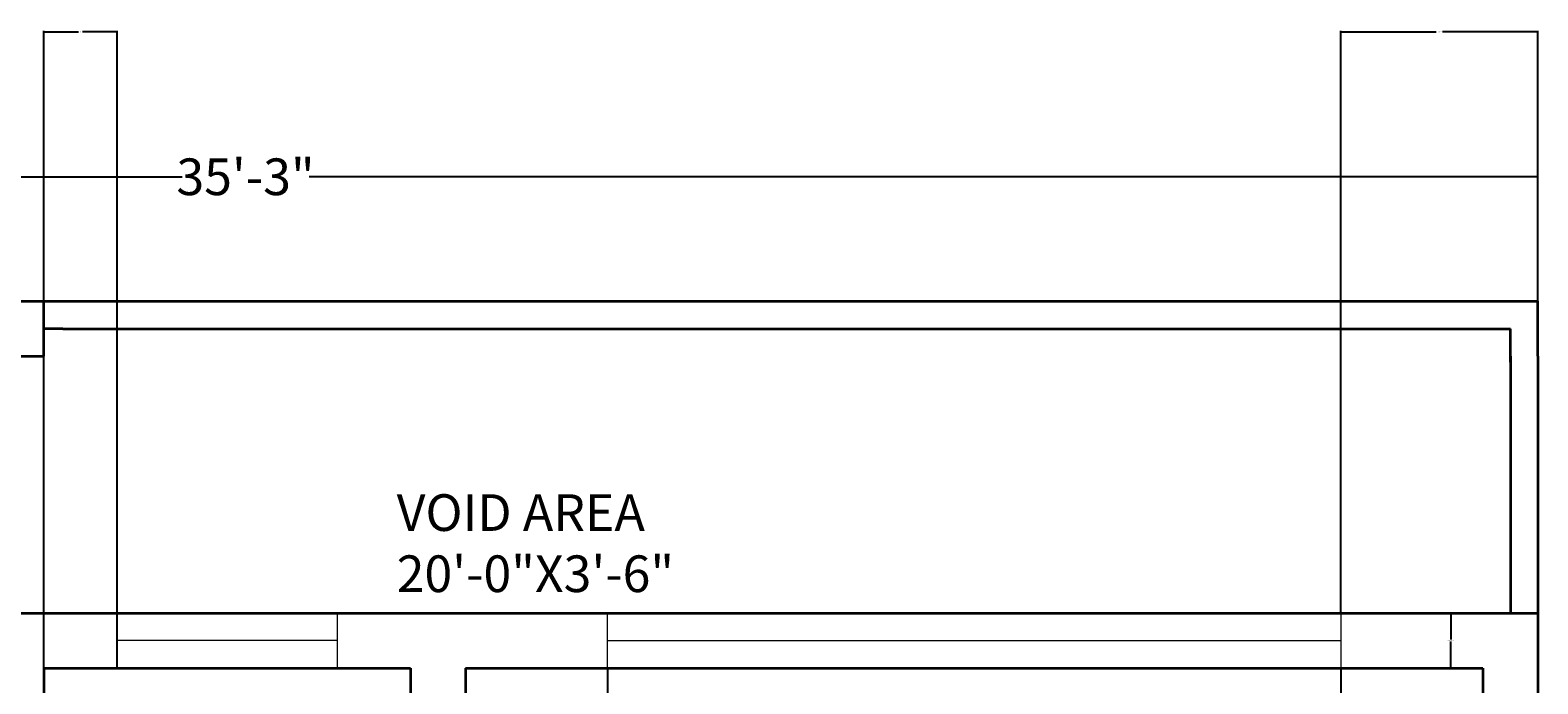
# Model space of a CAD drawing. Units: inches. Extents: x -10 to 502, y -868 to 56.
# Tile 14 of 14: x 211 to 458, y -50 to 56. Entities that reach past the tile are written whole.
import ezdxf

# ---------------------------------------------------------------- set-up
doc = ezdxf.new("R2010")
doc.units = ezdxf.units.IN
doc.header["$MEASUREMENT"] = 0
for name, color, linetype, lineweight in [('A-ANNO-DIMS', 2, 'Continuous', 18), ('A-AREA-IDEN', 7, 'Continuous', 18), ('A-GLAZ', 162, 'Continuous', 18), ('A-WALL', 7, 'Continuous', 35)]:
    doc.layers.add(name, color=color, linetype=linetype, lineweight=lineweight)
doc.styles.get("Standard").update_dxf_attribs({"font": 'arial.ttf'})
doc.dimstyles.get("Standard").update_dxf_attribs({"dimtxt": 0.18, "dimasz": 0.18, "dimexe": 0.18, "dimexo": 0.0625, "dimgap": 0.09, "dimtad": 0, "dimtih": 1, "dimtoh": 1, "dimdec": 0, "dimzin": 0, "dimdsep": 46, "dimlunit": 3, "dimtxsty": 'Standard', "dimcen": 0.09, "dimadec": 0, "dimazin": 0, "dimtfac": 1, "dimtdec": 0, "dimtofl": 0, "dimtmove": 0, "dimatfit": 3, "dimfxl": 1, "dimtolj": 1, "dimtzin": 0, "dimarcsym": 0})

# ---------------------------------------------------------------- blocks, each defined once
blk = doc.blocks.new('*D1')
at = {"layer": 'A-ANNO-DIMS', "color": 0, "lineweight": -2, "transparency": 16777216}
for p, q in [((34.95, 12.21), (34.95, 32.67)), ((35.13, 32.49), (236.06, 32.49)), ((457.77, 32.49), (256.84, 32.49)), ((457.95, 12.21), (457.95, 32.67))]:
    blk.add_line(p, q, dxfattribs=at)
at = {"layer": 'A-ANNO-DIMS', "color": 0, "transparency": 16777216}
for points in [[(35.13, 32.52), (35.13, 32.46), (34.95, 32.49)], [(457.77, 32.52), (457.77, 32.46), (457.95, 32.49)]]:
    blk.add_solid(points, dxfattribs=at)
at = {"layer": 'Defpoints', "color": 0, "transparency": 16777216}
for p in [(457.95, 32.49), (34.95, 12.15), (457.95, 12.15)]:
    blk.add_point(p, dxfattribs=at)
at = {"layer": 'A-ANNO-DIMS', "color": 0, "transparency": 16777216, "insert": (246.45, 32.49), "char_height": 6, "attachment_point": 5}
blk.add_mtext('\\A1;35\'-3"', dxfattribs=at)
blk = doc.blocks.new('WIN-36IN')
for p, q in [((0, 9), (36, 9)), ((0, 0), (0, 9)), ((36, 9), (36, 0)), ((0, 4.5), (36, 4.5)), ((36, 0), (0, 0))]:
    blk.add_line(p, q)
blk = doc.blocks.new('WIN-120IN')
for p, q in [((0, 9), (120, 9)), ((0, 0), (0, 9)), ((120, 9), (120, 0)), ((0, 4.5), (120, 4.5)), ((120, 0), (0, 0))]:
    blk.add_line(p, q)
blk = doc.blocks.new('*D21')
at = {"layer": 'A-ANNO-DIMS', "color": 0, "lineweight": -2, "transparency": 16777216}
for p, q in [((305.7, -47.92), (305.7, -66.03)), ((425.7, -47.92), (425.7, -66.03)), ((305.88, -65.85), (364.4, -65.85)), ((425.52, -65.85), (367, -65.85))]:
    blk.add_line(p, q, dxfattribs=at)
at = {"layer": 'A-ANNO-DIMS', "color": 0, "transparency": 16777216}
for points in [[(305.88, -65.82), (305.88, -65.88), (305.7, -65.85)], [(425.52, -65.82), (425.52, -65.88), (425.7, -65.85)]]:
    blk.add_solid(points, dxfattribs=at)
at = {"layer": 'Defpoints', "color": 0, "transparency": 16777216}
for p in [(305.7, -47.85), (425.7, -47.85), (425.7, -65.85)]:
    blk.add_point(p, dxfattribs=at)
at = {"layer": 'A-ANNO-DIMS', "color": 0, "transparency": 16777216, "insert": (365.7, -65.85), "char_height": 0.18, "attachment_point": 5}
blk.add_mtext('\\A1;WINDOW 10\'-0" TYP.', dxfattribs=at)
blk = doc.blocks.new('*D22')
at = {"layer": 'A-ANNO-DIMS', "color": 0, "lineweight": -2, "transparency": 16777216}
for p, q in [((425.76, -38.85), (443.88, -38.85)), ((443.7, -39.03), (443.7, -43.17)), ((443.7, -47.67), (443.7, -43.53)), ((425.76, -47.85), (443.88, -47.85))]:
    blk.add_line(p, q, dxfattribs=at)
at = {"layer": 'A-ANNO-DIMS', "color": 0, "transparency": 16777216}
for points in [[(443.67, -39.03), (443.73, -39.03), (443.7, -38.85)], [(443.67, -47.67), (443.73, -47.67), (443.7, -47.85)]]:
    blk.add_solid(points, dxfattribs=at)
at = {"layer": 'Defpoints', "color": 0, "transparency": 16777216}
for p in [(425.7, -38.85), (443.7, -38.85), (425.7, -47.85)]:
    blk.add_point(p, dxfattribs=at)
at = {"layer": 'A-ANNO-DIMS', "color": 0, "transparency": 16777216, "insert": (443.7, -43.35), "char_height": 0.18, "attachment_point": 5}
blk.add_mtext('\\A1;0\'-9" TYP.', dxfattribs=at)
blk = doc.blocks.new('*D50')
at = {"layer": 'A-ANNO-DIMS', "color": 0, "lineweight": -2, "transparency": 16777216}
for p, q in [((425.7, -38.79), (425.7, 56.38)), ((425.88, 56.2), (441.29, 56.2)), ((457.77, 56.2), (442.37, 56.2)), ((457.95, -38.79), (457.95, 56.38))]:
    blk.add_line(p, q, dxfattribs=at)
at = {"layer": 'A-ANNO-DIMS', "color": 0, "transparency": 16777216}
for points in [[(425.88, 56.23), (425.88, 56.17), (425.7, 56.2)], [(457.77, 56.23), (457.77, 56.17), (457.95, 56.2)]]:
    blk.add_solid(points, dxfattribs=at)
at = {"layer": 'Defpoints', "color": 0, "transparency": 16777216}
for p in [(457.95, 56.2), (425.7, -38.85), (457.95, -38.85)]:
    blk.add_point(p, dxfattribs=at)
at = {"layer": 'A-ANNO-DIMS', "color": 0, "transparency": 16777216, "insert": (441.83, 56.2), "char_height": 0.18, "attachment_point": 5}
blk.add_mtext('\\A1;2\'-8 1/2"', dxfattribs=at)
blk = doc.blocks.new('*D63')
at = {"layer": 'A-ANNO-DIMS', "color": 0, "lineweight": -2, "transparency": 16777216}
for p, q in [((213.45, -47.79), (213.45, 56.38)), ((213.63, 56.2), (219.13, 56.2)), ((225.27, 56.2), (219.77, 56.2)), ((225.45, -47.79), (225.45, 56.38))]:
    blk.add_line(p, q, dxfattribs=at)
at = {"layer": 'A-ANNO-DIMS', "color": 0, "transparency": 16777216}
for points in [[(213.63, 56.23), (213.63, 56.17), (213.45, 56.2)], [(225.27, 56.23), (225.27, 56.17), (225.45, 56.2)]]:
    blk.add_solid(points, dxfattribs=at)
at = {"layer": 'Defpoints', "color": 0, "transparency": 16777216}
for p in [(225.45, 56.2), (213.45, -47.85), (225.45, -47.85)]:
    blk.add_point(p, dxfattribs=at)
at = {"layer": 'A-ANNO-DIMS', "color": 0, "transparency": 16777216, "insert": (219.45, 56.2), "char_height": 0.18, "attachment_point": 5}
blk.add_mtext('\\A1;1\'-0"', dxfattribs=at)

msp = doc.modelspace()

# ---------------------------------------------------------------- linework, layer by layer
at = {"layer": 'A-WALL'}
for p, q in [((34.95, 12.15), (457.95, 12.15)), ((213.45, 3.15), (213.45, 12.15)), ((457.95, 3.15), (457.95, 12.15)), ((216.56, 7.65), (213.45, 7.65)), ((216.56, 7.65), (453.45, 7.65)), ((453.45, 2.15), (453.45, 7.65)), ((108.45, 3.15), (213.45, 3.15)), ((453.45, 3.15), (453.45, -38.85)), ((457.95, 3.15), (457.95, -770.85)), ((208.95, -38.85), (457.95, -38.85)), ((213.45, -47.85), (273.45, -47.85)), ((213.45, -47.85), (213.45, -143.85)), ((273.45, -47.85), (273.45, -143.85)), ((282.45, -47.85), (282.45, -227.85)), ((282.45, -47.85), (448.95, -47.85)), ((448.95, -47.85), (448.95, -254.85))]:
    msp.add_line(p, q, dxfattribs=at)

# ---------------------------------------------------------------- block references
at = {"layer": 'A-GLAZ', "rotation": 180}
msp.add_blockref('WIN-36IN', (261.45, -38.85), dxfattribs=at)
at = {"layer": 'A-GLAZ'}
msp.add_blockref('WIN-120IN', (305.7, -47.85), dxfattribs=at)

# ---------------------------------------------------------------- texts
at = {"layer": 'A-AREA-IDEN', "insert": (271.19, -19.43), "char_height": 6, "attachment_point": 1}
msp.add_mtext('VOID AREA\\P20\'-0"X3\'-6" ', dxfattribs=at)

# ---------------------------------------------------------------- dimensions: what is measured, and where the dimension line sits
at = {"layer": 'A-ANNO-DIMS'}
for base, p1, p2, override, picture, middle in [((225.45, 56.2), (213.45, -47.85), (225.45, -47.85), {"dimdec": 1, "dimlfac": 1, "dimrnd": 0, "dimzin": 1, "dimdsep": 46, "dimlunit": 4, "dimfrac": 2}, '*D63', (219.45, 56.2)), ((457.950916, 56.197263), (425.700916, -38.852737), (457.950916, -38.852737), {"dimdec": 1, "dimlfac": 1, "dimrnd": 0, "dimzin": 1, "dimdsep": 46, "dimlunit": 4, "dimfrac": 2}, '*D50', (441.825916, 56.197263)), ((457.95, 32.49), (34.95, 12.15), (457.95, 12.15), {"dimtxt": 6, "dimclrd": 0, "dimclre": 0, "dimclrt": 0}, '*D1', (246.45, 32.49))]:
    dim = msp.add_linear_dim(base=base, p1=p1, p2=p2, dimstyle='Standard', override=override, dxfattribs=at)
    dim.commit()
    dim.dimension.update_dxf_attribs({"geometry": picture, "text_midpoint": middle})
dim = msp.add_linear_dim(base=(443.7, -38.85), p1=(425.7, -47.85), p2=(425.7, -38.85), angle=90, text='<> TYP.', dimstyle='Standard', override={"dimdec": 1, "dimlfac": 1, "dimrnd": 0, "dimzin": 1, "dimdsep": 46, "dimlunit": 4, "dimfrac": 2}, dxfattribs=at)
dim.commit()
dim.dimension.update_dxf_attribs({"geometry": '*D22', "text_midpoint": (443.7, -43.35)})
dim = msp.add_linear_dim(base=(425.7, -65.85), p1=(305.7, -47.85), p2=(425.7, -47.85), text='WINDOW <> TYP.', dimstyle='Standard', override={"dimdec": 1, "dimlfac": 1, "dimrnd": 0, "dimzin": 1, "dimdsep": 46, "dimlunit": 4, "dimfrac": 2}, dxfattribs=at)
dim.commit()
dim.dimension.update_dxf_attribs({"geometry": '*D21', "text_midpoint": (365.7, -65.85)})

doc.saveas('drawing.dxf')
